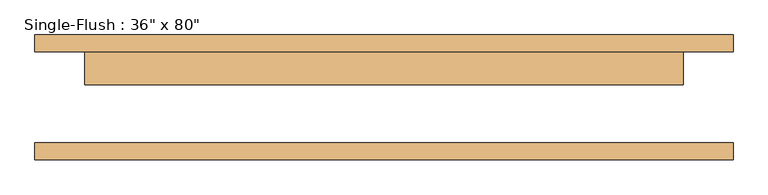
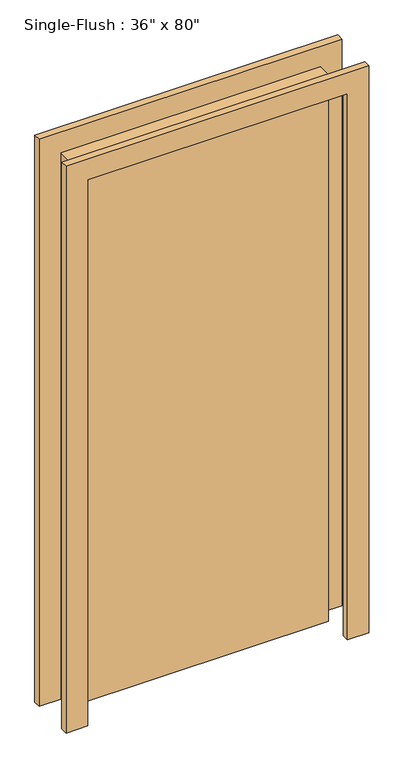
"""IFC4 building model written with IfcOpenShell, lengths in millimetres: door geometry."""

from ifc_helpers import new_model, si_unit, frame, origin, origin_with_axes, place, context, project, spatial, polyline, outline, extrude, source, transform, mapped, element, save


def door_ad1ac78c(model_context):
    return source(origin(), model_context, "Body", "SweptSolid", [
        extrude(outline(polyline([(2108.2, -533.4), (0.0, -533.4), (0.0, -457.2), (2032.0, -457.2), (2032.0, 457.2), (0.0, 457.2), (0.0, 533.4), (2108.2, 533.4), (2108.2, -533.4)])), frame((0.0, 69.85, 0.0), z_axis=(0.0, 1.0, 0.0), x_axis=(0.0, 0.0, 1.0)), (0.0, 0.0, 1.0), 25.4),
        extrude(outline(polyline([(2108.2, 533.4), (2108.2, -533.4), (0.0, -533.4), (0.0, -457.2), (2032.0, -457.2), (2032.0, 457.2), (0.0, 457.2), (0.0, 533.4), (2108.2, 533.4)])), frame((0.0, -95.25, 0.0), z_axis=(0.0, 1.0, 0.0), x_axis=(0.0, 0.0, 1.0)), (0.0, 0.0, 1.0), 25.4),
        extrude(outline(polyline([(457.2, 19.05), (-457.2, 19.05), (-457.2, 69.85), (457.2, 69.85), (457.2, 19.05)])), origin_with_axes(), (0.0, 0.0, 1.0), 2032.0),
    ])


if __name__ == "__main__":
    model = new_model("IFC4")
    model_context = context("Model", 3, world=origin())
    ifc_project = project(units=[si_unit("LENGTHUNIT", "METRE", prefix="MILLI")], contexts=[model_context])
    site = spatial("IfcSite", under=ifc_project)
    building = spatial("IfcBuilding", under=site)
    placement = place(None, origin())
    door_shape = door_ad1ac78c(model_context)
    element("IfcDoor", 1, ObjectType="Single-Flush : 36\" x 80\"", at=placement, inside=building, context=model_context, shape_type="MappedRepresentation", body=[
        mapped(door_shape, transform((0.0, 0.0, 0.0), x_axis=(1.0, 0.0, 0.0), y_axis=(0.0, 1.0, 0.0), z_axis=(0.0, 0.0, 1.0))),
    ])
    save(model, "model.ifc")

# Revit data of these elements
# Type "Single-Flush : 36\" x 80\""
#   Type Mark = "6"
#   Construction Type Id = "MDOOR"
#   Assembly Code = "C1020"
#   Analytic Construction = "Metal"
#   Thickness = 2"
#   Heat Transfer Coefficient (U) = 0.651978 BTU/(h·ft²·°F)
#   Height = 80"
#   Trim Projection Ext = 1"
#   Trim Projection Int = 1"
#   Trim Width = 3"
#   Width = 36"
#   Define Thermal Properties by = 1
#   Define Thermal Properties by = 1
#   Door Material = Door - Panel
#   Frame Material = Door - Frame
#   Visual Light Transmittance = 0
#   Solar Heat Gain Coefficient = 0
#   Function = (empty or 0)
#   Wall Closure = (empty or 0)
# Element 1 (IfcDoor, "Single-Flush : 36\" x 80\"")
#   Materials on its faces: "Door - Frame", "Door - Panel"
# Materials
#   "Door - Panel": class "Wood", colour RGB 210 159 95, transparency 0, Cost = 0
#   "Door - Frame": colour RGB 118 70 51, transparency 0, Cost = 0
